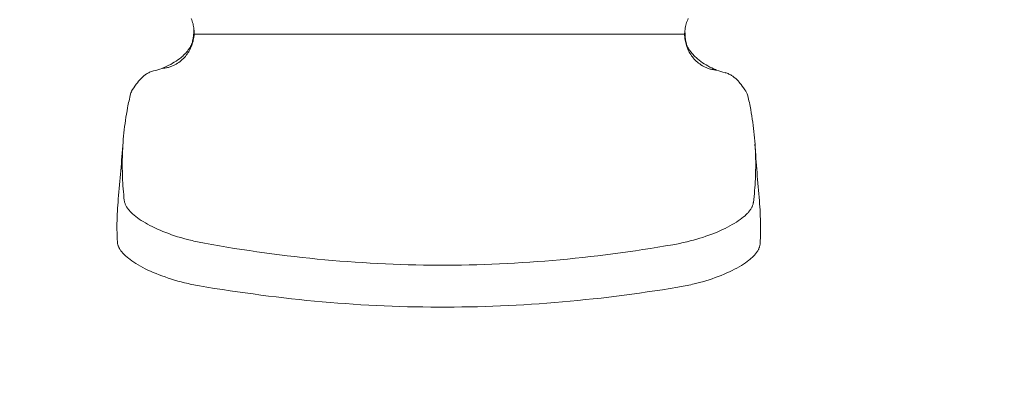
# Model space of a CAD drawing. Units: inches. Extents: x -466983 to 1020, y 324 to 318697.
# Tile 33 of 97: x 847.81 to 867.6, y 734.38 to 741.85. Entities that reach past the tile are written whole.
import ezdxf

# ---------------------------------------------------------------- set-up
doc = ezdxf.new("R2010")
doc.units = ezdxf.units.IN
doc.header["$MEASUREMENT"] = 0
for name, color, linetype, lineweight in [('A-ANNO-DIMS', 2, 'Continuous', 18), ('A-FLOR-PATT', 252, 'Continuous', 13), ('A-FURN', 8, 'Continuous', 18)]:
    doc.layers.add(name, color=color, linetype=linetype, lineweight=lineweight)
doc.styles.get("Standard").update_dxf_attribs({"font": 'arial.ttf'})
doc.dimstyles.get("Standard").update_dxf_attribs({"dimtxt": 6, "dimasz": 4, "dimexe": 3, "dimexo": 3, "dimgap": 0.09, "dimtad": 0, "dimtih": 1, "dimtoh": 1, "dimdec": 1, "dimzin": 0, "dimdsep": 46, "dimlunit": 3, "dimtxsty": 'Standard', "dimcen": 0.09, "dimadec": 0, "dimazin": 0, "dimtfac": 1, "dimtdec": 1, "dimtofl": 0, "dimtmove": 0, "dimatfit": 3, "dimfxl": 1, "dimtolj": 1, "dimtzin": 0, "dimarcsym": 0})

# ---------------------------------------------------------------- blocks, each defined once
blk = doc.blocks.new('Office Chairs')
at = {"ltscale": 60}
for p, q in [((2665.7, 922.3), (2666.3, 920.9)), ((2666.3, 920.9), (2666.8, 919.5)), ((2666.8, 919.5), (2667.2, 918.1)), ((2667.2, 918.1), (2667.6, 916.6)), ((3184.3, 917.9), (3183.8, 916.5)), ((3184.8, 919.3), (3184.3, 917.9)), ((3185.4, 920.7), (3184.8, 919.3)), ((3186, 922.1), (3185.4, 920.7)), ((2667.6, 916.6), (2667.9, 915.2)), ((2667.9, 915.2), (2668.2, 913.8)), ((2668.2, 913.8), (2668.4, 912.4)), ((2668.4, 912.4), (2668.6, 910.9)), ((2668.6, 910.9), (2668.7, 909.5)), ((2668.7, 909.8), (2668.6, 905.9)), ((2668.7, 909.5), (2668.7, 908.1)), ((2668.7, 908.1), (2668.7, 907.4)), ((2668.7, 907.4), (2668.7, 907.3)), ((3182.3, 907.9), (3182.2, 906.5)), ((3182.4, 909.4), (3182.3, 907.9)), ((3182.3, 908.4), (3182.3, 904.3)), ((3182.6, 910.8), (3182.4, 909.4)), ((3182.8, 912.2), (3182.6, 910.8)), ((3183.1, 913.7), (3182.8, 912.2)), ((3183.4, 915.1), (3183.1, 913.7)), ((3183.8, 916.5), (3183.4, 915.1)), ((2666.7, 896.5), (2666.9, 897.3)), ((2666.7, 895.4), (2667.2, 896.8)), ((2666.9, 897.3), (2667.1, 898.3)), ((2667.1, 898.3), (2667.2, 898.5)), ((2667.2, 898.5), (2667.2, 898.5)), ((2667.2, 896.8), (2667.6, 898.2)), ((2667.6, 898.2), (2667.9, 899.6)), ((2667.9, 899.6), (2668.2, 901.1)), ((2668.2, 901.1), (2668.4, 902.5)), ((2668.4, 902.5), (2668.6, 904)), ((2668.6, 905.9), (2668.6, 904.7)), ((2668.6, 904), (2668.6, 904.7)), ((3182.2, 906.5), (3182.2, 905.8)), ((3182.3, 904.3), (3182.3, 903.2)), ((3182.4, 902.4), (3182.3, 903.2)), ((3182.5, 901), (3182.4, 902.4)), ((3182.7, 899.5), (3182.5, 901)), ((3183, 898.1), (3182.7, 899.5)), ((3183.3, 896.6), (3183, 898.1)), ((3183.8, 896.6), (3183.7, 896.9)), ((3183.7, 896.9), (3183.7, 896.9)), ((2660.6, 886.8), (2659.9, 886)), ((2661.3, 887.6), (2660.6, 886.8)), ((2662, 888.5), (2661.3, 887.6)), ((2662.6, 889.3), (2662, 888.5)), ((2662.3, 886.1), (2663.1, 887.4)), ((2663.3, 890.2), (2662.6, 889.3)), ((2663.1, 887.4), (2663.8, 888.7)), ((2663.9, 891.1), (2663.3, 890.2)), ((2663.8, 888.7), (2664.5, 890)), ((2664.5, 892), (2663.9, 891.1)), ((2665, 893), (2664.5, 892)), ((2664.5, 890), (2665.1, 891.3)), ((2665.5, 894), (2665, 893)), ((2665.1, 891.3), (2665.7, 892.6)), ((2666, 894.9), (2665.5, 894)), ((2665.7, 892.6), (2666.3, 894)), ((2666.5, 895.9), (2666, 894.9)), ((2666.3, 894), (2666.7, 895.4)), ((2666.5, 895.9), (2666.7, 896.5)), ((3183.7, 895.2), (3183.3, 896.6)), ((3184.1, 893.8), (3183.7, 895.2)), ((3184, 895.7), (3183.8, 896.6)), ((3184.2, 894.9), (3184, 895.7)), ((3184.6, 892.4), (3184.1, 893.8)), ((3184.4, 894.3), (3184.2, 894.9)), ((3184.4, 894.3), (3184.9, 893.3)), ((3185.2, 891), (3184.6, 892.4)), ((3184.9, 893.3), (3185.3, 892.3)), ((3185.7, 889.7), (3185.2, 891)), ((3185.3, 892.3), (3185.9, 891.4)), ((3186.4, 888.4), (3185.7, 889.7)), ((3185.9, 891.4), (3186.4, 890.4)), ((3186.4, 890.4), (3187, 889.5)), ((3187.1, 887.1), (3186.4, 888.4)), ((3187, 889.5), (3187.6, 888.6)), ((3187.8, 885.8), (3187.1, 887.1)), ((3187.6, 888.6), (3188.2, 887.7)), ((3188.2, 887.7), (3188.9, 886.9)), ((3188.9, 886.9), (3189.6, 886)), ((2648, 876.4), (2646.2, 875.3)), ((2649.9, 877.6), (2648, 876.4)), ((2651.7, 878.8), (2649.9, 877.6)), ((2651.4, 875.3), (2652.8, 876.2)), ((2653.4, 880.1), (2651.7, 878.8)), ((2652.8, 876.2), (2654.1, 877.2)), ((2655.1, 881.5), (2653.4, 880.1)), ((2654.1, 877.2), (2655.3, 878.2)), ((2656, 882.2), (2655.1, 881.5)), ((2655.3, 878.2), (2656.4, 879.2)), ((2656.8, 882.9), (2656, 882.2)), ((2656.4, 879.2), (2657.5, 880.3)), ((2657.6, 883.7), (2656.8, 882.9)), ((2657.5, 880.3), (2658.6, 881.4)), ((2658.4, 884.4), (2657.6, 883.7)), ((2659.1, 885.2), (2658.4, 884.4)), ((2658.6, 881.4), (2659.6, 882.6)), ((2659.9, 886), (2659.1, 885.2)), ((2659.6, 882.6), (2660.5, 883.7)), ((2660.5, 883.7), (2661.4, 884.9)), ((2661.4, 884.9), (2662.3, 886.1)), ((3188.6, 884.5), (3187.8, 885.8)), ((3189.4, 883.3), (3188.6, 884.5)), ((3190.3, 882.1), (3189.4, 883.3)), ((3189.6, 886), (3190.3, 885.2)), ((3190.3, 885.2), (3191, 884.4)), ((3191.2, 880.9), (3190.3, 882.1)), ((3191, 884.4), (3191.7, 883.6)), ((3192.2, 879.8), (3191.2, 880.9)), ((3191.7, 883.6), (3192.5, 882.8)), ((3193.3, 878.7), (3192.2, 879.8)), ((3192.5, 882.8), (3193.3, 882)), ((3193.3, 882), (3194.1, 881.3)), ((3194.4, 877.6), (3193.3, 878.7)), ((3194.1, 881.3), (3194.9, 880.6)), ((3195.5, 876.5), (3194.4, 877.6)), ((3194.9, 880.6), (3195.7, 879.9)), ((3196.7, 875.5), (3195.5, 876.5)), ((3195.7, 879.9), (3197.4, 878.5)), ((3197.4, 878.5), (3199.1, 877.2)), ((3199.1, 877.2), (3200.9, 875.9)), ((2621.2, 865.5), (2622.1, 865.9)), ((2622.1, 865.9), (2623.1, 866.3)), ((2623.1, 866.3), (2624.1, 866.7)), ((2624.1, 866.7), (2625.1, 867.1)), ((2625.1, 867.1), (2626.2, 867.3)), ((2626.2, 867.3), (2626.2, 867.3)), ((2636.2, 870.4), (2635.1, 870)), ((2635.1, 870), (2636.1, 870.1)), ((2636.1, 870.1), (2637.1, 870.2)), ((2638.2, 871.3), (2636.2, 870.4)), ((2637.1, 870.2), (2638.1, 870.3)), ((2638.1, 870.3), (2639, 870.4)), ((2640.3, 872.2), (2638.2, 871.3)), ((2639, 870.4), (2640, 870.6)), ((2640, 870.6), (2640.9, 870.8)), ((2642.3, 873.2), (2640.3, 872.2)), ((2640.9, 870.8), (2641.8, 871)), ((2641.8, 871), (2642.7, 871.3)), ((2644.2, 874.2), (2642.3, 873.2)), ((2642.7, 871.3), (2643.6, 871.6)), ((2643.6, 871.6), (2644.5, 871.9)), ((2646.2, 875.3), (2644.2, 874.2)), ((2644.5, 871.9), (2645.3, 872.2)), ((2645.3, 872.2), (2646.2, 872.5)), ((2646.2, 872.5), (2647, 872.9)), ((2647, 872.9), (2647.8, 873.2)), ((2647.8, 873.2), (2648.5, 873.6)), ((2648.5, 873.6), (2650, 874.4)), ((2650, 874.4), (2651.4, 875.3)), ((3198, 874.6), (3196.7, 875.5)), ((3199.3, 873.6), (3198, 874.6)), ((3200.8, 872.8), (3199.3, 873.6)), ((3202.2, 871.9), (3200.8, 872.8)), ((3200.9, 875.9), (3202.7, 874.7)), ((3203, 871.5), (3202.2, 871.9)), ((3202.7, 874.7), (3204.6, 873.6)), ((3203.8, 871.2), (3203, 871.5)), ((3204.6, 870.8), (3203.8, 871.2)), ((3204.6, 873.6), (3206.5, 872.5)), ((3205.4, 870.5), (3204.6, 870.8)), ((3206.3, 870.2), (3205.4, 870.5)), ((3207.1, 869.9), (3206.3, 870.2)), ((3206.5, 872.5), (3208.5, 871.4)), ((3208, 869.6), (3207.1, 869.9)), ((3208.9, 869.3), (3208, 869.6)), ((3208.5, 871.4), (3210.5, 870.5)), ((3209.8, 869.1), (3208.9, 869.3)), ((3210.7, 868.9), (3209.8, 869.1)), ((3210.5, 870.5), (3212.5, 869.5)), ((3211.7, 868.7), (3210.7, 868.9)), ((3212.7, 868.5), (3211.7, 868.7)), ((3212.5, 869.5), (3214.6, 868.7)), ((3213.6, 868.4), (3212.7, 868.5)), ((3214.6, 868.3), (3213.6, 868.4)), ((3214.6, 868.7), (3215.6, 868.3)), ((3215.6, 868.3), (3214.6, 868.3)), ((2609.3, 854.9), (2610.6, 856.5)), ((2610.6, 856.5), (2611.5, 857.6)), ((2611.5, 857.6), (2612.5, 858.7)), ((2612.5, 858.7), (2613.5, 859.8)), ((2613.5, 859.8), (2614.7, 860.9)), ((2614.7, 860.9), (2615.9, 862)), ((2615.9, 862), (2616.6, 862.5)), ((2616.6, 862.5), (2617.2, 863)), ((2617.2, 863), (2618, 863.6)), ((2618, 863.6), (2618.7, 864.1)), ((2618.7, 864.1), (2619.5, 864.6)), ((2619.5, 864.6), (2620.3, 865)), ((2620.3, 865), (2621.2, 865.5)), ((3224.5, 865.5), (3224.5, 865.5)), ((3225.6, 865.2), (3224.5, 865.5)), ((3226.6, 864.9), (3225.6, 865.2)), ((3227.6, 864.5), (3226.6, 864.9)), ((3228.6, 864.1), (3227.6, 864.5)), ((3229.5, 863.7), (3228.6, 864.1)), ((3230.4, 863.2), (3229.5, 863.7)), ((3231.2, 862.7), (3230.4, 863.2)), ((3232, 862.2), (3231.2, 862.7)), ((3232.7, 861.7), (3232, 862.2)), ((3233.4, 861.2), (3232.7, 861.7)), ((3234.1, 860.6), (3233.4, 861.2)), ((3234.8, 860.1), (3234.1, 860.6)), ((3236, 859), (3234.8, 860.1)), ((3237.1, 857.9), (3236, 859)), ((3238.2, 856.8), (3237.1, 857.9)), ((3239.2, 855.7), (3238.2, 856.8)), ((3240.1, 854.6), (3239.2, 855.7)), ((2603.7, 846.7), (2603.6, 846.6)), ((2603.7, 846.7), (2604.4, 847.9)), ((2604.4, 847.9), (2605.5, 849.6)), ((2605.5, 849.6), (2606.7, 851.5)), ((2606.7, 851.5), (2608.1, 853.4)), ((2608.1, 853.4), (2609.3, 854.9)), ((3241.3, 853), (3240.1, 854.6)), ((3242.5, 851.5), (3241.3, 853)), ((3243.9, 849.5), (3242.5, 851.5)), ((3245.1, 847.7), (3243.9, 849.5)), ((3246.2, 846), (3245.1, 847.7)), ((3246.9, 844.8), (3246.2, 846)), ((3246.9, 844.8), (3246.9, 844.6)), ((2597.9, 822.2), (2598.5, 825.5)), ((2598.5, 825.5), (2599.1, 828.8)), ((3251.9, 823.6), (3251.4, 826.9)), ((2596.4, 812.3), (2596.9, 815.6)), ((2596.9, 815.6), (2597.4, 818.9)), ((2597.4, 818.9), (2597.9, 822.2)), ((3252.5, 820.2), (3251.9, 823.6)), ((3253, 816.9), (3252.5, 820.2)), ((3253.5, 813.6), (3253, 816.9)), ((2595.2, 802.4), (2595.6, 805.7)), ((2595.6, 805.7), (2596, 809)), ((2596, 809), (2596.4, 812.3)), ((3253.9, 810.3), (3253.5, 813.6)), ((3254.3, 807), (3253.9, 810.3)), ((3254.7, 803.8), (3254.3, 807)), ((2594.3, 792.5), (2594.6, 795.8)), ((2594.6, 795.8), (2594.9, 799.1)), ((2594.9, 799.1), (2595.2, 802.4)), ((3255.1, 800.5), (3254.7, 803.8)), ((3255.4, 797.2), (3255.1, 800.5)), ((3255.6, 793.9), (3255.4, 797.2)), ((3255.9, 790.6), (3255.6, 793.9)), ((2593.7, 780.4), (2593.8, 783.4)), ((2593.8, 783.4), (2594, 786.4)), ((2594, 786.4), (2594.1, 789.5)), ((2594.1, 789.5), (2594.3, 792.5)), ((3256.1, 787.6), (3255.9, 790.6)), ((3256.2, 784.5), (3256.1, 787.6)), ((3256.4, 781.5), (3256.2, 784.5)), ((2593.5, 774.3), (2593.6, 777.4)), ((2593.5, 771.3), (2593.5, 774.3)), ((2593.6, 777.4), (2593.7, 780.4)), ((3256.5, 778.5), (3256.4, 781.5)), ((3256.5, 775.4), (3256.5, 778.5)), ((3256.6, 772.4), (3256.5, 775.4)), ((2593.5, 768.3), (2593.5, 771.3)), ((2593.5, 765.3), (2593.5, 768.3)), ((2593.6, 762.2), (2593.5, 765.3)), ((3256.5, 763.3), (3256.6, 766.4)), ((3256.5, 760.3), (3256.5, 763.3)), ((3256.6, 769.4), (3256.6, 772.4)), ((3256.6, 766.4), (3256.6, 769.4)), ((2593.6, 759.2), (2593.6, 762.2)), ((2593.7, 756.2), (2593.6, 759.2)), ((2593.9, 753.1), (2593.7, 756.2)), ((2594, 750.1), (2593.9, 753.1)), ((3256.1, 751.1), (3256.2, 754.2)), ((3256.2, 754.2), (3256.4, 757.2)), ((3256.4, 757.2), (3256.5, 760.3)), ((2594.2, 747), (2594, 750.1)), ((2594.5, 744), (2594.2, 747)), ((2594.7, 740.9), (2594.5, 744)), ((3255.4, 742), (3255.7, 745)), ((3255.7, 745), (3255.9, 748.1)), ((3255.9, 748.1), (3256.1, 751.1)), ((2589.1, 730.1), (2589.4, 733.3)), ((2595, 737.8), (2594.7, 740.9)), ((2595.3, 734.8), (2595, 737.8)), ((2595.6, 731.7), (2595.3, 734.8)), ((3254.2, 729.7), (3254.6, 732.8)), ((3254.6, 732.8), (3254.9, 735.9)), ((3254.9, 735.9), (3255.2, 738.9)), ((3255.2, 738.9), (3255.4, 742)), ((2588.5, 720.5), (2588.6, 723.7)), ((2588.6, 723.7), (2588.9, 726.9)), ((2588.9, 726.9), (2589.1, 730.1)), ((2595.6, 731.7), (2595.7, 731.1)), ((2595.7, 731.1), (2595.8, 730.4)), ((2595.8, 730.4), (2596, 729.8)), ((2596, 729.8), (2596.2, 729.2)), ((2596.2, 729.2), (2596.4, 728.5)), ((2596.4, 728.5), (2596.6, 727.9)), ((2596.6, 727.9), (2596.9, 727.2)), ((2596.9, 727.2), (2597.2, 726.6)), ((2597.2, 726.6), (2597.6, 725.9)), ((2597.6, 725.9), (2598, 725.2)), ((2598, 725.2), (2598.4, 724.6)), ((2598.4, 724.6), (2598.8, 723.9)), ((2598.8, 723.9), (2599.3, 723.2)), ((2599.3, 723.2), (2599.8, 722.5)), ((2599.8, 722.5), (2600.4, 721.9)), ((2600.4, 721.9), (2601, 721.2)), ((3250.9, 721.9), (3250.4, 721.2)), ((3251.4, 722.6), (3250.9, 721.9)), ((3251.8, 723.2), (3251.4, 722.6)), ((3252.2, 723.9), (3251.8, 723.2)), ((3252.5, 724.6), (3252.2, 723.9)), ((3252.9, 725.2), (3252.5, 724.6)), ((3253.2, 725.9), (3252.9, 725.2)), ((3253.4, 726.5), (3253.2, 725.9)), ((3253.6, 727.2), (3253.4, 726.5)), ((3253.8, 727.8), (3253.6, 727.2)), ((3254, 728.4), (3253.8, 727.8)), ((3254.1, 729.1), (3254, 728.4)), ((3254.2, 729.7), (3254.1, 729.1)), ((3260.7, 728.2), (3260.4, 731.4)), ((3260.9, 725), (3260.7, 728.2)), ((3261.1, 721.8), (3260.9, 725)), ((3261.3, 718.5), (3261.1, 721.8)), ((2588.1, 710.8), (2588.2, 714.1)), ((2588.2, 714.1), (2588.3, 717.3)), ((2588.3, 717.3), (2588.5, 720.5)), ((2601, 721.2), (2601.6, 720.5)), ((2601.6, 720.5), (2602.2, 719.8)), ((2602.2, 719.8), (2602.9, 719.1)), ((2602.9, 719.1), (2603.6, 718.5)), ((2603.6, 718.5), (2604.3, 717.8)), ((2604.3, 717.8), (2605.9, 716.4)), ((2605.9, 716.4), (2607.6, 715)), ((2607.6, 715), (2609.4, 713.6)), ((2609.4, 713.6), (2611.3, 712.3)), ((2611.3, 712.3), (2613.3, 710.9)), ((3240.3, 711.7), (3238.4, 710.4)), ((3242.1, 713.1), (3240.3, 711.7)), ((3243.8, 714.5), (3242.1, 713.1)), ((3245.4, 715.8), (3243.8, 714.5)), ((3246.1, 716.5), (3245.4, 715.8)), ((3246.8, 717.2), (3246.1, 716.5)), ((3247.5, 717.9), (3246.8, 717.2)), ((3248.2, 718.5), (3247.5, 717.9)), ((3248.8, 719.2), (3248.2, 718.5)), ((3249.4, 719.9), (3248.8, 719.2)), ((3249.9, 720.6), (3249.4, 719.9)), ((3250.4, 721.2), (3249.9, 720.6)), ((3261.4, 715.3), (3261.3, 718.5)), ((3261.5, 712.1), (3261.4, 715.3)), ((3261.6, 708.9), (3261.5, 712.1)), ((2588, 707.6), (2588.1, 710.8)), ((2588, 704.4), (2588, 707.6)), ((2588, 701.2), (2588, 704.4)), ((2588.1, 698), (2588, 701.2)), ((2613.3, 710.9), (2615.5, 709.6)), ((2615.5, 709.6), (2617.7, 708.2)), ((2617.7, 708.2), (2620, 706.9)), ((2620, 706.9), (2622.5, 705.6)), ((2622.5, 705.6), (2625, 704.3)), ((2625, 704.3), (2627.7, 703)), ((2627.7, 703), (2630.4, 701.7)), ((2630.4, 701.7), (2633.2, 700.5)), ((3222, 701.2), (3219.2, 699.9)), ((3224.6, 702.5), (3222, 701.2)), ((3227.1, 703.7), (3224.6, 702.5)), ((3229.6, 705), (3227.1, 703.7)), ((3232, 706.4), (3229.6, 705)), ((3234.2, 707.7), (3232, 706.4)), ((3236.4, 709), (3234.2, 707.7)), ((3238.4, 710.4), (3236.4, 709)), ((3261.6, 705.6), (3261.6, 708.9)), ((3261.6, 702.4), (3261.6, 705.6)), ((3261.6, 699.2), (3261.6, 702.4)), ((2588.1, 694.7), (2588.1, 698)), ((2588.3, 691.5), (2588.1, 694.7)), ((2588.4, 688.2), (2588.3, 691.5)), ((2633.2, 700.5), (2636.1, 699.3)), ((2636.1, 699.3), (2639, 698.1)), ((2639, 698.1), (2642.1, 697)), ((2642.1, 697), (2645.2, 695.9)), ((2645.2, 695.9), (2648.3, 694.8)), ((2648.3, 694.8), (2651.5, 693.8)), ((2651.5, 693.8), (2654.8, 692.8)), ((2654.8, 692.8), (2658.1, 691.8)), ((2658.1, 691.8), (2661.5, 690.9)), ((2661.5, 690.9), (2664.8, 690)), ((3194.8, 691.1), (3191.4, 690.2)), ((3198, 692.1), (3194.8, 691.1)), ((3201.3, 693.1), (3198, 692.1)), ((3204.4, 694.2), (3201.3, 693.1)), ((3207.5, 695.3), (3204.4, 694.2)), ((3210.6, 696.4), (3207.5, 695.3)), ((3213.5, 697.5), (3210.6, 696.4)), ((3216.4, 698.7), (3213.5, 697.5)), ((3219.2, 699.9), (3216.4, 698.7)), ((3261.3, 689.5), (3261.5, 692.7)), ((3261.5, 695.9), (3261.6, 699.2)), ((3261.5, 692.7), (3261.5, 695.9)), ((2588.4, 687.6), (2588.4, 688.2)), ((2588.5, 687), (2588.4, 687.6)), ((2588.6, 686.3), (2588.5, 687)), ((2588.8, 685.6), (2588.6, 686.3)), ((2589, 685), (2588.8, 685.6)), ((2589.2, 684.3), (2589, 685)), ((2589.5, 683.7), (2589.2, 684.3)), ((2589.8, 683), (2589.5, 683.7)), ((2590.1, 682.3), (2589.8, 683)), ((2590.5, 681.6), (2590.1, 682.3)), ((2590.8, 680.9), (2590.5, 681.6)), ((2591.3, 680.3), (2590.8, 680.9)), ((2591.7, 679.6), (2591.3, 680.3)), ((2687.4, 685.5), (2679.5, 686.9)), ((2695.2, 684.2), (2687.4, 685.5)), ((2703, 682.9), (2695.2, 684.2)), ((2710.9, 681.6), (2703, 682.9)), ((2718.7, 680.4), (2710.9, 681.6)), ((2726.6, 679.2), (2718.7, 680.4)), ((3130.8, 679.1), (3138.6, 680.3)), ((3138.6, 680.3), (3146.5, 681.5)), ((3146.5, 681.5), (3154.3, 682.8)), ((3154.3, 682.8), (3162.2, 684.1)), ((3162.2, 684.1), (3170, 685.4)), ((3188.1, 689.3), (3184.7, 688.4)), ((3191.4, 690.2), (3188.1, 689.3)), ((3259.1, 679.6), (3259.4, 680.3)), ((3259.4, 680.3), (3259.8, 680.9)), ((3259.8, 680.9), (3260, 681.6)), ((3260, 681.6), (3260.3, 682.3)), ((3260.3, 682.3), (3260.5, 682.9)), ((3260.5, 682.9), (3260.7, 683.6)), ((3260.7, 683.6), (3260.9, 684.3)), ((3260.9, 684.3), (3261, 684.9)), ((3261, 684.9), (3261.1, 685.6)), ((3261.1, 685.6), (3261.2, 686.2)), ((3261.2, 686.2), (3261.3, 689.5)), ((2592.2, 678.9), (2591.7, 679.6)), ((2592.8, 678.2), (2592.2, 678.9)), ((2593.3, 677.5), (2592.8, 678.2)), ((2593.9, 676.8), (2593.3, 677.5)), ((2594.6, 676.1), (2593.9, 676.8)), ((2595.2, 675.4), (2594.6, 676.1)), ((2595.9, 674.7), (2595.2, 675.4)), ((2596.7, 674), (2595.9, 674.7)), ((2597.4, 673.3), (2596.7, 674)), ((2598.2, 672.6), (2597.4, 673.3)), ((2599, 671.9), (2598.2, 672.6)), ((2599.9, 671.2), (2599, 671.9)), ((2601.7, 669.8), (2599.9, 671.2)), ((2734.4, 678), (2726.6, 679.2)), ((2742.3, 676.9), (2734.4, 678)), ((2750.2, 675.9), (2742.3, 676.9)), ((2758.1, 674.9), (2750.2, 675.9)), ((2766, 673.9), (2758.1, 674.9)), ((2773.9, 672.9), (2766, 673.9)), ((2781.8, 672.1), (2773.9, 672.9)), ((2789.7, 671.2), (2781.8, 672.1)), ((2797.6, 670.4), (2789.7, 671.2)), ((2805.5, 669.7), (2797.6, 670.4)), ((3051.8, 669.6), (3059.7, 670.4)), ((3059.7, 670.4), (3067.7, 671.2)), ((3067.7, 671.2), (3075.6, 672)), ((3075.6, 672), (3083.5, 672.9)), ((3083.5, 672.9), (3091.4, 673.8)), ((3091.4, 673.8), (3099.3, 674.8)), ((3099.3, 674.8), (3107.1, 675.8)), ((3107.1, 675.8), (3115, 676.9)), ((3115, 676.9), (3122.9, 678)), ((3122.9, 678), (3130.8, 679.1)), ((3249.5, 669.2), (3250.4, 669.9)), ((3250.4, 669.9), (3251.2, 670.6)), ((3251.2, 670.6), (3252, 671.3)), ((3252, 671.3), (3252.8, 672)), ((3252.8, 672), (3253.5, 672.7)), ((3253.5, 672.7), (3254.2, 673.4)), ((3254.2, 673.4), (3254.9, 674.1)), ((3254.9, 674.1), (3255.5, 674.8)), ((3255.5, 674.8), (3256.1, 675.5)), ((3256.1, 675.5), (3256.7, 676.2)), ((3256.7, 676.2), (3257.2, 676.9)), ((3257.2, 676.9), (3257.7, 677.6)), ((3257.7, 677.6), (3258.2, 678.2)), ((3258.2, 678.2), (3258.7, 678.9)), ((3258.7, 678.9), (3259.1, 679.6)), ((2603.6, 668.4), (2601.7, 669.8)), ((2605.7, 667), (2603.6, 668.4)), ((2607.8, 665.6), (2605.7, 667)), ((2610.1, 664.3), (2607.8, 665.6)), ((2612.5, 662.9), (2610.1, 664.3)), ((2615, 661.5), (2612.5, 662.9)), ((2617.6, 660.2), (2615, 661.5)), ((2620.3, 658.9), (2617.6, 660.2)), ((2813.4, 668.9), (2805.5, 669.7)), ((2821.4, 668.3), (2813.4, 668.9)), ((2829.3, 667.7), (2821.4, 668.3)), ((2837.2, 667.1), (2829.3, 667.7)), ((2845.2, 666.6), (2837.2, 667.1)), ((2853.1, 666.1), (2845.2, 666.6)), ((2861.1, 665.7), (2853.1, 666.1)), ((2869, 665.3), (2861.1, 665.7)), ((2877, 664.9), (2869, 665.3)), ((2884.9, 664.7), (2877, 664.9)), ((2892.9, 664.4), (2884.9, 664.7)), ((2900.8, 664.2), (2892.9, 664.4)), ((2908.8, 664.1), (2900.8, 664.2)), ((2916.7, 664), (2908.8, 664.1)), ((2924.7, 663.9), (2916.7, 664)), ((2924.7, 663.9), (2932.7, 663.9)), ((2932.7, 663.9), (2940.6, 664)), ((2940.6, 664), (2948.6, 664.1)), ((2948.6, 664.1), (2956.5, 664.2)), ((2956.5, 664.2), (2964.5, 664.4)), ((2964.5, 664.4), (2972.4, 664.7)), ((2972.4, 664.7), (2980.4, 664.9)), ((2980.4, 664.9), (2988.3, 665.3)), ((2988.3, 665.3), (2996.3, 665.7)), ((2996.3, 665.7), (3004.2, 666.1)), ((3004.2, 666.1), (3012.2, 666.6)), ((3012.2, 666.6), (3020.1, 667.1)), ((3020.1, 667.1), (3028, 667.7)), ((3028, 667.7), (3036, 668.3)), ((3036, 668.3), (3043.9, 668.9)), ((3043.9, 668.9), (3051.8, 669.6)), ((3231.8, 658.3), (3234.4, 659.7)), ((3234.4, 659.7), (3236.9, 661)), ((3236.9, 661), (3239.3, 662.3)), ((3239.3, 662.3), (3241.6, 663.7)), ((3241.6, 663.7), (3243.7, 665.1)), ((3243.7, 665.1), (3245.8, 666.5)), ((3245.8, 666.5), (3247.7, 667.8)), ((3247.7, 667.8), (3249.5, 669.2)), ((2623.1, 657.6), (2620.3, 658.9)), ((2626, 656.3), (2623.1, 657.6)), ((2628.9, 655.1), (2626, 656.3)), ((2632, 653.9), (2628.9, 655.1)), ((2635.1, 652.7), (2632, 653.9)), ((2638.3, 651.6), (2635.1, 652.7)), ((2641.6, 650.5), (2638.3, 651.6)), ((2644.9, 649.4), (2641.6, 650.5)), ((2648.3, 648.4), (2644.9, 649.4)), ((3207.7, 648.7), (3211, 649.8)), ((3211, 649.8), (3214.2, 651)), ((3214.2, 651), (3217.4, 652.1)), ((3217.4, 652.1), (3220.4, 653.3)), ((3220.4, 653.3), (3223.4, 654.5)), ((3223.4, 654.5), (3226.3, 655.8)), ((3226.3, 655.8), (3229.1, 657)), ((3229.1, 657), (3231.8, 658.3)), ((2651.8, 647.4), (2648.3, 648.4)), ((2655.2, 646.5), (2651.8, 647.4)), ((2658.8, 645.6), (2655.2, 646.5)), ((2682.2, 641), (2674.2, 642.4)), ((2690.2, 639.7), (2682.2, 641)), ((2698.3, 638.4), (2690.2, 639.7)), ((3159, 638.3), (3167, 639.6)), ((3167, 639.6), (3175, 640.9)), ((3190.5, 644), (3194, 644.8)), ((3194, 644.8), (3197.5, 645.7)), ((3197.5, 645.7), (3201, 646.7)), ((3201, 646.7), (3204.4, 647.7)), ((3204.4, 647.7), (3207.7, 648.7)), ((2706.3, 637.2), (2698.3, 638.4)), ((2714.3, 636), (2706.3, 637.2)), ((2722.3, 634.9), (2714.3, 636)), ((2730.4, 633.8), (2722.3, 634.9)), ((2738.4, 632.7), (2730.4, 633.8)), ((2746.5, 631.6), (2738.4, 632.7)), ((2754.5, 630.7), (2746.5, 631.6)), ((2762.6, 629.7), (2754.5, 630.7)), ((2770.6, 628.8), (2762.6, 629.7)), ((2778.7, 627.9), (2770.6, 628.8)), ((3078.5, 627.9), (3086.6, 628.7)), ((3086.6, 628.7), (3094.7, 629.6)), ((3094.7, 629.6), (3102.7, 630.6)), ((3102.7, 630.6), (3110.8, 631.5)), ((3110.8, 631.5), (3118.8, 632.6)), ((3118.8, 632.6), (3126.9, 633.6)), ((3126.9, 633.6), (3134.9, 634.7)), ((3134.9, 634.7), (3143, 635.9)), ((3143, 635.9), (3151, 637.1)), ((3151, 637.1), (3159, 638.3)), ((2786.8, 627.1), (2778.7, 627.9)), ((2794.9, 626.3), (2786.8, 627.1)), ((2802.9, 625.6), (2794.9, 626.3)), ((2811, 624.9), (2802.9, 625.6)), ((2819.1, 624.3), (2811, 624.9)), ((2827.2, 623.7), (2819.1, 624.3)), ((2835.3, 623.1), (2827.2, 623.7)), ((2843.4, 622.6), (2835.3, 623.1)), ((2851.5, 622.2), (2843.4, 622.6)), ((2859.6, 621.7), (2851.5, 622.2)), ((2867.7, 621.4), (2859.6, 621.7)), ((2875.9, 621), (2867.7, 621.4)), ((2884, 620.8), (2875.9, 621)), ((2892.1, 620.5), (2884, 620.8)), ((2900.2, 620.3), (2892.1, 620.5)), ((2908.3, 620.2), (2900.2, 620.3)), ((2916.4, 620.1), (2908.3, 620.2)), ((2924.6, 620.1), (2916.4, 620.1)), ((2924.6, 620.1), (2932.7, 620.1)), ((2932.7, 620.1), (2940.8, 620.1)), ((2940.8, 620.1), (2948.9, 620.2)), ((2948.9, 620.2), (2957, 620.3)), ((2957, 620.3), (2965.2, 620.5)), ((2965.2, 620.5), (2973.3, 620.7)), ((2973.3, 620.7), (2981.4, 621)), ((2981.4, 621), (2989.5, 621.3)), ((2989.5, 621.3), (2997.6, 621.7)), ((2997.6, 621.7), (3005.7, 622.1)), ((3005.7, 622.1), (3013.8, 622.6)), ((3013.8, 622.6), (3021.9, 623.1)), ((3021.9, 623.1), (3030, 623.6)), ((3030, 623.6), (3038.1, 624.2)), ((3038.1, 624.2), (3046.2, 624.9)), ((3046.2, 624.9), (3054.3, 625.6)), ((3054.3, 625.6), (3062.4, 626.3)), ((3062.4, 626.3), (3070.5, 627.1)), ((3070.5, 627.1), (3078.5, 627.9))]:
    blk.add_line(p, q, dxfattribs=at)
for centre, radius, start, end in [((2513.8, 922.9), 155.3, 350.9637, 355.404), ((2630.8, 907.6), 38, 355.6747, 359.5543), ((3337.3, 920.4), 155.4, 184.2192, 188.7233), ((2641.2, 906.8), 27.5, 336.7908, 355.7382), ((3220.2, 905.8), 38, 179.9955, 183.9737), ((3209.7, 905), 27.5, 183.9105, 202.9229), ((2609.6, 938.7), 73.3, 283.1123, 290.4025), ((3241.6, 936.8), 73.3, 249.248, 256.539), ((2635.1, 831.8), 34.8, 156.9535, 160.7468), ((2626.8, 833.6), 26.6, 150.734, 153.5115), ((2889.1, 774.1), 295.1, 166.4415, 169.3107), ((3223.7, 831.8), 26.5, 26.1158, 28.8961), ((3215.5, 830.1), 34.7, 18.8733, 22.6726), ((2961.1, 774.1), 295, 10.3061, 13.1763), ((-314.3, 1005.7), 2916.4, 354.6406, 355.8078), ((6165.8, 985.7), 2916.5, 183.8367, 185.0032), ((2720.5, 915.1), 231.8, 256.1178, 259.8291), ((3130.4, 913.9), 231.9, 279.8227, 283.5334), ((2713.5, 871.9), 232.9, 256.4051, 260.2856), ((3137.1, 870.7), 232.9, 279.3662, 283.2462)]:
    blk.add_arc(centre, radius, start, end, dxfattribs=at)
blk.add_arc((3250.5, 2757372.8), 2756467, 269.9879058, 269.9985896)
blk = doc.blocks.new('Office Desk With Chairs')
at = {"xscale": 0.0191941550942558, "yscale": 0.0191941550942558, "zscale": 0.0191941550942558}
blk.add_blockref('Office Chairs', (2012.509, 1014.21), dxfattribs=at)
blk = doc.blocks.new('*D99')
at = {"layer": 'A-ANNO-DIMS', "color": 0, "lineweight": -2, "transparency": 16777216}
for p, q in [((833.84, 822.679), (820.85, 822.679)), ((823.85, 818.679), (823.85, 782.572)), ((823.85, 740.077), (823.85, 776.184)), ((833.84, 736.077), (820.85, 736.077))]:
    blk.add_line(p, q, dxfattribs=at)
at = {"layer": 'A-ANNO-DIMS', "color": 0, "transparency": 16777216}
for points in [[(823.183, 818.679), (824.517, 818.679), (823.85, 822.679)], [(823.183, 740.077), (824.517, 740.077), (823.85, 736.077)]]:
    blk.add_solid(points, dxfattribs=at)
at = {"layer": 'Defpoints', "color": 0, "transparency": 16777216}
for p in [(823.85, 822.679), (836.84, 822.679), (836.84, 736.077)]:
    blk.add_point(p, dxfattribs=at)
at = {"layer": 'A-ANNO-DIMS', "color": 0, "transparency": 16777216, "insert": (823.85, 779.378), "char_height": 6, "attachment_point": 5}
blk.add_mtext('\\A1;OFFICE DESK 87', dxfattribs=at)

msp = doc.modelspace()

# ---------------------------------------------------------------- hatches: boundary and pattern name
at = {"layer": 'A-FLOR-PATT', "transparency": 33554572}
h = msp.add_hatch(dxfattribs=at)
h.set_pattern_fill('ANSI37', color=256, scale=30)
h.set_pattern_definition([(45, (-1212.4137, -290.035), (-2.6516504, 2.6516504), []), (135, (-1212.4137, -290.035), (-2.6516504, -2.6516504), [])])
h.paths.add_polyline_path([(901.806, 1075.938), (900.614, 1075.938), (900.614, 1065.386), (899.391, 1065.386), (898.091, 1065.386), (892.836, 1058.71, -0.258377), (892.188, 1058.351), (879.985, 1058.351, -0.20177), (879.438, 1058.581), (874.081, 1065.386), (872.781, 1065.386), (871.558, 1065.386), (871.558, 1075.938), (813.806, 1075.938), (813.806, 1044.792), (832.395, 1044.792, -0.394795), (848.66, 1028.536), (848.66, 1009.938), (901.806, 1009.938), (901.806, 1015.938), (901.306, 1015.938), (871.306, 1015.938), (871.306, 1017.25), (871.334, 1017.25, -0.401453), (901.306, 1045.938), (901.806, 1045.938)])
edge = h.paths.add_edge_path(flags=16)
edge.add_line((847.773, 1068.949), (847.773, 1073.709))
edge.add_arc((849.227, 1073.709), 1.454, 90, 180, ccw=False)
edge.add_line((849.227, 1075.163), (864.492, 1075.163))
edge.add_arc((864.492, 1073.709), 1.454, 0, 90, ccw=False)
edge.add_line((865.946, 1073.709), (865.946, 1069.004))
edge.add_arc((832.645, 1068.976), 33.301, -20.6123, 0.0472, ccw=False)
edge.add_ellipse((856.859, 1058.48), major_axis=(0, 10.213), ratio=0.685919, start_angle=100.0088, end_angle=259.9912, ccw=False)
edge.add_arc((881.074, 1068.976), 33.301, 180.0472, 200.6123, ccw=False)
h.paths.add_polyline_path([(853.146, 1066.482), (853.146, 1066.453), (853.146, 1066.453, 0.433107), (852.917, 1066.685), (852.917, 1066.453), (853.146, 1066.453), (853.146, 1066.482), (853.088, 1066.612, 0.697939), (852.7, 1066.453), (852.7, 1066.453), (852.7, 1066.482), (852.917, 1067.001), (852.917, 1066.685, -0.396254)], flags=0)
h.paths.add_polyline_path([(861.019, 1066.482), (861.019, 1066.453), (861.019, 1066.453, 0.416404), (860.802, 1066.685), (860.802, 1066.453), (861.019, 1066.453), (861.019, 1066.482), (860.967, 1066.605, 0.713344), (860.573, 1066.453), (860.573, 1066.453), (860.573, 1066.482), (860.802, 1067.001), (860.802, 1066.685, -0.379973)], flags=0)
edge = h.paths.add_edge_path(flags=0)
edge.add_spline(control_points=[(861.13, 1065.785), (861.466, 1065.248), (861.613, 1065.016), (861.983, 1064.374), (862.192, 1063.944), (862.561, 1063.039), (862.721, 1062.563), (862.987, 1061.578), (863.092, 1061.069), (863.245, 1060.031), (863.293, 1059.503), (863.329, 1058.441), (863.318, 1057.908), (863.237, 1056.852), (863.166, 1056.329), (862.97, 1055.308), (862.843, 1054.81), (862.537, 1053.852), (862.357, 1053.393), (861.951, 1052.525), (861.725, 1052.117), (861.233, 1051.362), (860.967, 1051.016), (860.405, 1050.395), (860.108, 1050.12), (859.494, 1049.646), (859.176, 1049.448), (858.528, 1049.13), (858.197, 1049.011), (857.531, 1048.852), (857.196, 1048.812), (856.525, 1048.812), (856.189, 1048.852), (855.524, 1049.01), (855.193, 1049.129), (854.545, 1049.447), (854.227, 1049.645), (853.612, 1050.118), (853.316, 1050.393), (852.753, 1051.014), (852.487, 1051.36), (851.995, 1052.114), (851.769, 1052.523), (851.363, 1053.39), (851.183, 1053.85), (850.877, 1054.807), (850.75, 1055.305), (850.553, 1056.326), (850.483, 1056.849), (850.401, 1057.905), (850.39, 1058.438), (850.426, 1059.5), (850.473, 1060.028), (850.626, 1061.066), (850.732, 1061.575), (850.997, 1062.561), (851.157, 1063.036), (851.525, 1063.942), (851.734, 1064.371), (852.106, 1065.016), (852.254, 1065.25), (852.608, 1065.733)], knot_values=[3.915332, 3.915332, 3.915332, 3.915332, 4.013468, 4.013468, 4.175532, 4.175532, 4.337596, 4.337596, 4.49966, 4.49966, 4.661724, 4.661724, 4.823788, 4.823788, 4.985852, 4.985852, 5.147916, 5.147916, 5.30998, 5.30998, 5.472044, 5.472044, 5.634109, 5.634109, 5.796173, 5.796173, 5.958237, 5.958237, 6.120301, 6.120301, 6.282365, 6.282365, 6.444429, 6.444429, 6.606493, 6.606493, 6.768557, 6.768557, 6.930621, 6.930621, 7.092685, 7.092685, 7.254749, 7.254749, 7.416813, 7.416813, 7.578878, 7.578878, 7.740942, 7.740942, 7.903006, 7.903006, 8.06507, 8.06507, 8.227134, 8.227134, 8.389198, 8.389198, 8.551262, 8.551262, 8.65037, 8.65037, 8.65037, 8.65037], degree=3, periodic=0)
edge.add_line((852.642, 1065.785), (861.13, 1065.785))
edge = h.paths.add_edge_path(flags=0)
edge.add_ellipse((856.85, 1057.743), major_axis=(0, 7.792), ratio=0.687861, start_angle=0, end_angle=360)
h.paths.add_polyline_path([(848.863, 1069.389), (848.863, 1073.96, -0.414214), (849.954, 1075.051), (863.765, 1075.051, -0.414214), (864.856, 1073.96), (864.856, 1069.389, -0.388936), (864.524, 1069.027, -0.043561), (849.195, 1069.027, -0.388936)], flags=0)
h.paths.add_polyline_path([(853.101, 1068.112, -1), (852.677, 1068.112, -1)], flags=0)
edge = h.paths.add_edge_path(flags=0)
edge.add_ellipse((856.859, 1057.338), major_axis=(0, 2.207), ratio=0.657164, start_angle=0, end_angle=360)
h.paths.add_polyline_path([(861.041, 1068.112, -1), (860.618, 1068.112, -1)], flags=0)
edge = h.paths.add_edge_path()
edge.add_line((573.954, 1057.341), (573.954, 1075.938))
edge.add_line((573.954, 1075.938), (558.731, 1075.938))
edge.add_line((558.731, 1075.938), (558.731, 1065.386))
edge.add_line((558.731, 1065.386), (557.507, 1065.386))
edge.add_line((557.507, 1065.386), (556.207, 1065.386))
edge.add_line((556.207, 1065.386), (550.952, 1058.71))
edge.add_arc((550.304, 1059.116), 0.765, 270, 327.9483, ccw=False)
edge.add_line((550.304, 1058.351), (538.101, 1058.351))
edge.add_arc((538.101, 1059.116), 0.765, 224.3704, 270, ccw=False)
edge.add_line((537.555, 1058.581), (532.198, 1065.386))
edge.add_line((532.198, 1065.386), (530.898, 1065.386))
edge.add_line((530.898, 1065.386), (529.674, 1065.386))
edge.add_line((529.674, 1065.386), (529.674, 1075.938))
edge.add_line((529.674, 1075.938), (520.806, 1075.938))
edge.add_line((520.806, 1075.938), (520.806, 1045.938))
edge.add_line((520.806, 1045.938), (521.306, 1045.938))
edge.add_arc((521.306, 1015.938), 30, 2.5075, 90, ccw=False)
edge.add_line((551.277, 1017.25), (551.306, 1017.25))
edge.add_line((551.306, 1017.25), (551.306, 1015.938))
edge.add_line((551.306, 1015.938), (520.806, 1015.938))
edge.add_line((520.806, 1015.938), (520.806, 1009.938))
edge.add_line((520.806, 1009.938), (559.191, 1010.402))
edge.add_arc((559.191, 1011.856), 1.454, 180, 270, ccw=False)
edge.add_line((557.737, 1011.856), (557.737, 1016.561))
edge.add_arc((591.039, 1016.589), 33.301, 159.3877, 180.0472, ccw=False)
edge.add_ellipse((566.824, 1027.085), major_axis=(0, 10.213), ratio=0.685919, start_angle=280.0088, end_angle=439.9912, ccw=False)
edge.add_arc((542.609, 1016.589), 33.301, 0.0472, 20.6123, ccw=False)
edge.add_line((575.91, 1016.616), (575.91, 1011.856))
edge.add_arc((574.456, 1011.856), 1.454, -90, 0, ccw=False)
edge.add_line((574.456, 1010.402), (608.806, 1009.938))
edge.add_line((608.806, 1009.938), (608.806, 1041.086))
edge.add_line((608.806, 1041.086), (590.218, 1041.086))
edge.add_arc((590.775, 1057.907), 16.831, 181.9277, 268.1032, ccw=False)
edge = h.paths.add_edge_path()
edge.add_ellipse((494.244, 583.62), major_axis=(0, 10.213), ratio=0.685919, start_angle=280.0088, end_angle=439.9912, ccw=False)
edge.add_arc((470.03, 573.124), 33.301, 0.0472, 20.6123, ccw=False)
edge.add_line((503.331, 573.152), (503.331, 568.392))
edge.add_arc((501.877, 568.392), 1.454, -90, 0, ccw=False)
edge.add_line((501.877, 566.938), (539.806, 566.938))
edge.add_line((539.806, 566.938), (539.806, 572.938))
edge.add_line((539.806, 572.938), (539.306, 572.938))
edge.add_line((539.306, 572.938), (509.306, 572.938))
edge.add_line((509.306, 572.938), (509.306, 574.25))
edge.add_line((509.306, 574.25), (509.334, 574.25))
edge.add_arc((539.306, 572.938), 30, 90, 177.4925, ccw=False)
edge.add_line((539.306, 602.938), (539.806, 602.938))
edge.add_line((539.806, 602.938), (539.806, 626.938))
edge.add_line((539.806, 626.938), (531.772, 626.938))
edge.add_line((531.772, 626.938), (531.772, 616.386))
edge.add_line((531.772, 616.386), (530.548, 616.386))
edge.add_line((530.548, 616.386), (529.249, 616.386))
edge.add_line((529.249, 616.386), (523.711, 609.351))
edge.add_line((523.711, 609.351), (510.777, 609.351))
edge.add_line((510.777, 609.351), (505.239, 616.386))
edge.add_line((505.239, 616.386), (503.939, 616.386))
edge.add_line((503.939, 616.386), (502.715, 616.386))
edge.add_line((502.715, 616.386), (502.715, 626.938))
edge.add_line((502.715, 626.938), (481.698, 626.938))
edge.add_line((481.698, 626.938), (481.698, 610.995))
edge.add_arc((467.27, 611.473), 14.436, 271.9277, 358.1032, ccw=False)
edge.add_line((467.756, 597.045), (451.806, 597.045))
edge.add_line((451.806, 597.045), (451.806, 584.404))
edge.add_line((451.806, 584.404), (451.806, 566.938))
edge.add_line((451.806, 566.938), (486.612, 566.938))
edge.add_arc((486.612, 568.392), 1.454, 180, 270, ccw=False)
edge.add_line((485.158, 568.392), (485.158, 573.097))
edge.add_arc((518.459, 573.124), 33.301, 159.3877, 180.0472, ccw=False)
h.paths.add_polyline_path([(836.261, 1020.733), (879.89, 1020.733), (879.89, 1039.39), (836.261, 1039.39)], flags=25)
h.paths.add_polyline_path([(549.985, 1036.749), (593.614, 1036.749), (593.614, 1055.407), (549.985, 1055.407)], flags=24)
h.paths.add_polyline_path([(475.123, 595.596), (518.752, 595.596), (518.752, 614.253), (475.123, 614.253)], flags=24)

# ---------------------------------------------------------------- block references
at = {"layer": 'A-FURN'}
msp.add_blockref('Office Desk With Chairs', (-1212.414, -290.035), dxfattribs=at)

# ---------------------------------------------------------------- dimensions: what is measured, and where the dimension line sits
at = {"layer": 'A-ANNO-DIMS'}
dim = msp.add_linear_dim(base=(823.85, 822.679), p1=(836.84, 736.077), p2=(836.84, 822.679), angle=90, text='OFFICE DESK <>', dimstyle='Standard', override={"dimdec": 0, "dimlfac": 1, "dimrnd": 0, "dimzin": 0, "dimdsep": 46, "dimlunit": 2}, dxfattribs=at)
dim.commit()
dim.dimension.update_dxf_attribs({"geometry": '*D99', "text_midpoint": (823.85, 779.378)})

doc.saveas('drawing.dxf')
